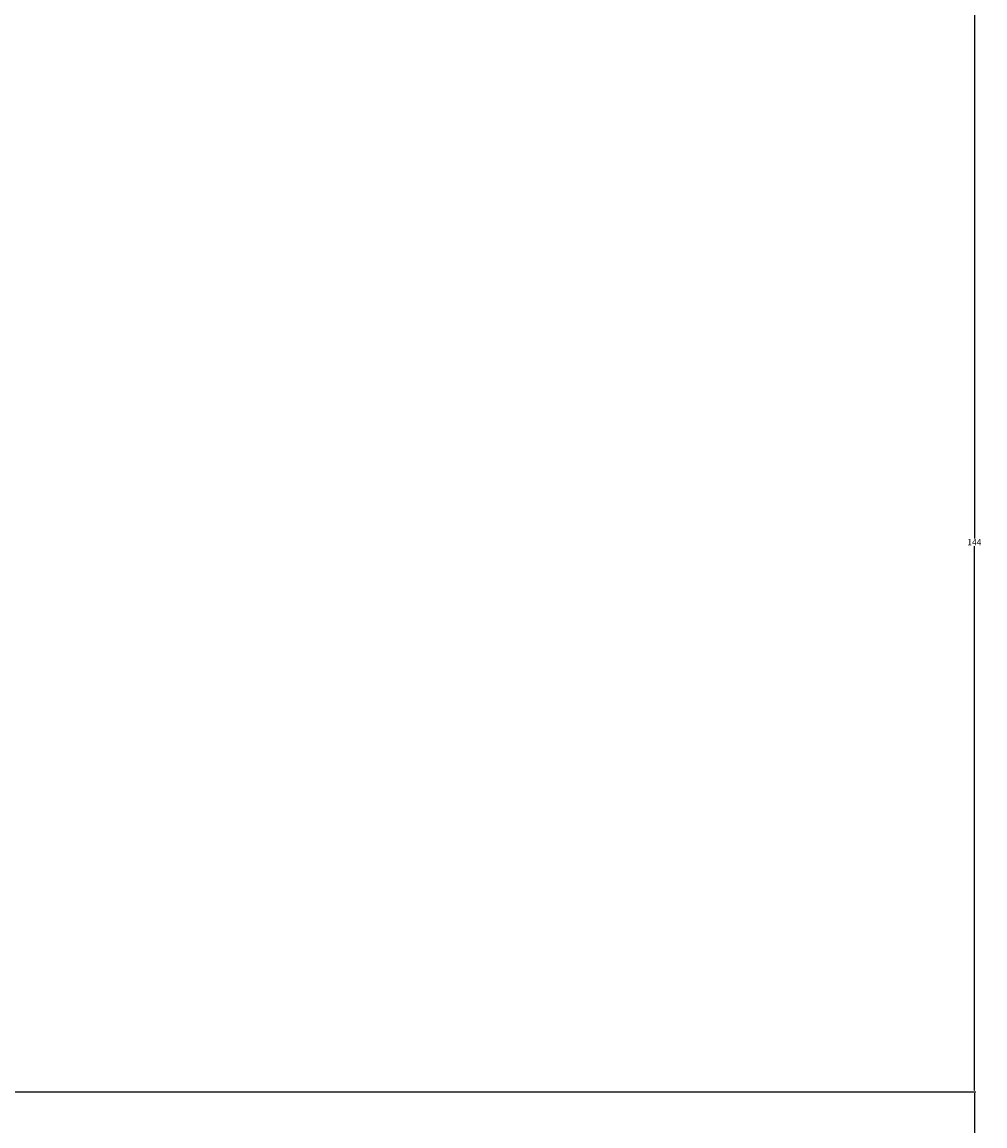
# Model space of a CAD drawing. Units: inches. Extents: x 36 to 594, y 79 to 831.
# Tile 26 of 30: x 468 to 594, y 446 to 590. Entities that reach past the tile are written whole.
import ezdxf

# ---------------------------------------------------------------- set-up
doc = ezdxf.new("R2010")
doc.units = ezdxf.units.IN
doc.header["$MEASUREMENT"] = 0
doc.layers.add('A-ANNO-DIMS', color=2, linetype='Continuous', lineweight=18)
doc.styles.get("Standard").update_dxf_attribs({"font": 'arial.ttf'})
doc.dimstyles.get("Standard").update_dxf_attribs({"dimtxt": 0.8125, "dimasz": 0.18, "dimexe": 0.18, "dimexo": 0.0625, "dimgap": 0.09, "dimtad": 0, "dimtih": 1, "dimtoh": 1, "dimdec": 4, "dimzin": 0, "dimdsep": 46, "dimlunit": 4, "dimtxsty": 'Standard', "dimcen": 0.09, "dimadec": 0, "dimazin": 0, "dimtfac": 1, "dimtdec": 4, "dimtofl": 0, "dimtmove": 0, "dimatfit": 3, "dimfxl": 1, "dimtolj": 1, "dimtzin": 0, "dimarcsym": 0})

# ---------------------------------------------------------------- blocks, each defined once
blk = doc.blocks.new('*D34')
at = {"layer": 'A-ANNO-DIMS', "color": 0, "lineweight": -2, "transparency": 16777216}
for p, q in [((448.45, 450.21), (592.85, 450.21)), ((592.67, 450.03), (592.67, 438.48)), ((592.67, 425.91), (592.67, 437.47)), ((424.61, 425.73), (592.85, 425.73))]:
    blk.add_line(p, q, dxfattribs=at)
at = {"layer": 'A-ANNO-DIMS', "color": 0, "transparency": 16777216}
for points in [[(592.64, 450.03), (592.7, 450.03), (592.67, 450.21)], [(592.64, 425.91), (592.7, 425.91), (592.67, 425.73)]]:
    blk.add_solid(points, dxfattribs=at)
at = {"layer": 'Defpoints', "color": 0, "transparency": 16777216}
for p in [(448.39, 450.21), (592.67, 450.21), (424.55, 425.73)]:
    blk.add_point(p, dxfattribs=at)
at = {"layer": 'A-ANNO-DIMS', "color": 0, "transparency": 16777216, "insert": (592.67, 437.97), "char_height": 0.812, "attachment_point": 5}
blk.add_mtext('\\A1;24.48', dxfattribs=at)
blk = doc.blocks.new('*D35')
at = {"layer": 'A-ANNO-DIMS', "color": 0, "lineweight": -2, "transparency": 16777216}
for p, q in [((424.56, 594.21), (592.85, 594.21)), ((592.67, 594.03), (592.67, 522.71)), ((592.67, 450.39), (592.67, 521.71)), ((448.45, 450.21), (592.85, 450.21))]:
    blk.add_line(p, q, dxfattribs=at)
at = {"layer": 'A-ANNO-DIMS', "color": 0, "transparency": 16777216}
for points in [[(592.64, 594.03), (592.7, 594.03), (592.67, 594.21)], [(592.64, 450.39), (592.7, 450.39), (592.67, 450.21)]]:
    blk.add_solid(points, dxfattribs=at)
at = {"layer": 'Defpoints', "color": 0, "transparency": 16777216}
for p in [(424.5, 594.21), (592.67, 594.21), (448.39, 450.21)]:
    blk.add_point(p, dxfattribs=at)
at = {"layer": 'A-ANNO-DIMS', "color": 0, "transparency": 16777216, "insert": (592.67, 522.21), "char_height": 0.812, "attachment_point": 5}
blk.add_mtext('\\A1;144', dxfattribs=at)

msp = doc.modelspace()

# ---------------------------------------------------------------- dimensions: what is measured, and where the dimension line sits
at = {"layer": 'A-ANNO-DIMS'}
for base, p1, p2, override, picture, middle in [((592.6689, 594.2124), (448.3898, 450.2124), (424.4958, 594.2124), {"dimdec": 0, "dimlfac": 1, "dimrnd": 0, "dimzin": 0, "dimdsep": 46, "dimlunit": 2}, '*D35', (592.6689, 522.2124)), ((592.6689, 450.2124), (424.5492, 425.7333), (448.3898, 450.2124), {"dimdec": 2, "dimlfac": 1, "dimrnd": 0, "dimzin": 0, "dimdsep": 46, "dimlunit": 2}, '*D34', (592.6689, 437.9728))]:
    dim = msp.add_linear_dim(base=base, p1=p1, p2=p2, angle=90, dimstyle='Standard', override=override, dxfattribs=at)
    dim.commit()
    dim.dimension.update_dxf_attribs({"geometry": picture, "text_midpoint": middle})

doc.saveas('drawing.dxf')
